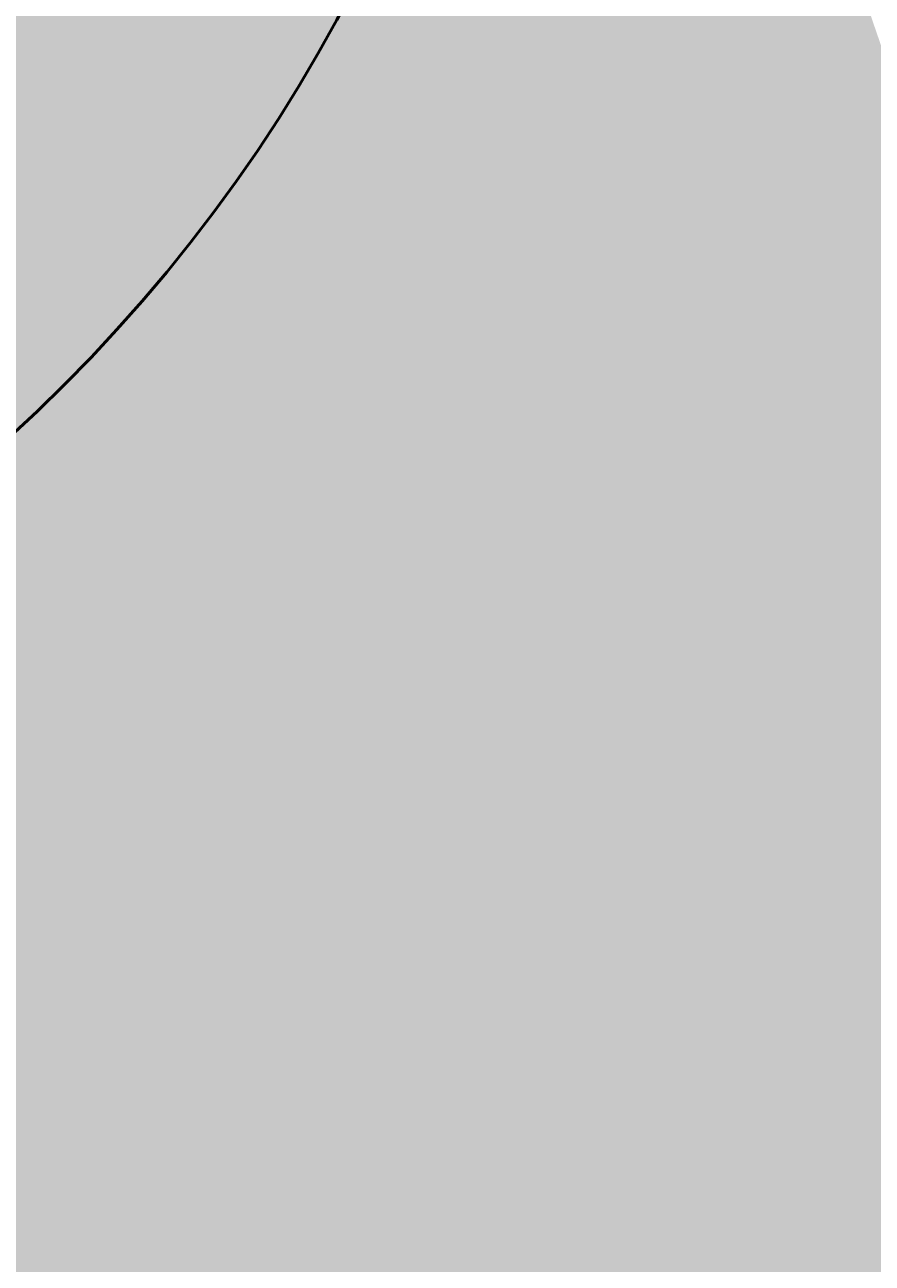
# Model space of a CAD drawing. Units: inches. Extents: x 114 to 236, y -51 to 115.
# Tile 10 of 14: x 196 to 212, y 41 to 65. Entities that reach past the tile are written whole.
import ezdxf

# ---------------------------------------------------------------- set-up
doc = ezdxf.new("R2010")
doc.units = ezdxf.units.IN
doc.header["$MEASUREMENT"] = 0
doc.layers.add('M-DIMS', color=2, linetype='Continuous', lineweight=18)
doc.layers.add('M-OUTL', color=7, linetype='Continuous', lineweight=50)
doc.layers.add('M-HATC', color=7, linetype='Continuous', lineweight=18, true_color=0xffffff)
doc.styles.get("Standard").update_dxf_attribs({"font": 'arial.ttf'})
doc.dimstyles.get("Standard").update_dxf_attribs({"dimtxt": 0.18, "dimasz": 0.18, "dimexe": 0.18, "dimexo": 0.0625, "dimgap": 0.09, "dimtad": 0, "dimtih": 1, "dimtoh": 1, "dimdec": 4, "dimzin": 0, "dimdsep": 46, "dimtxsty": 'Standard', "dimcen": 0.09, "dimadec": 0, "dimazin": 0, "dimtfac": 1, "dimtdec": 4, "dimtofl": 0, "dimtmove": 0, "dimatfit": 3, "dimfxl": 1, "dimtolj": 1, "dimtzin": 0, "dimarcsym": 0})

# ---------------------------------------------------------------- blocks, each defined once
blk = doc.blocks.new('*D3')
at = {"layer": 'Defpoints', "color": 0, "transparency": 16777216}
for p in [(230.229, 115.287), (120.229, 9.307), (230.229, 9.307)]:
    blk.add_point(p, dxfattribs=at)
at = {"layer": 'M-DIMS', "color": 0, "lineweight": -2, "transparency": 16777216}
for p, q in [((120.229, 9.37), (120.229, 115.467)), ((120.409, 115.287), (174.949, 115.287)), ((230.049, 115.287), (175.509, 115.287)), ((230.229, 9.37), (230.229, 115.467))]:
    blk.add_line(p, q, dxfattribs=at)
at = {"layer": 'M-DIMS', "color": 0, "transparency": 16777216}
for points in [[(120.409, 115.317), (120.409, 115.257), (120.229, 115.287)], [(230.049, 115.317), (230.049, 115.257), (230.229, 115.287)]]:
    blk.add_solid(points, dxfattribs=at)
at = {"layer": 'M-DIMS', "color": 0, "transparency": 16777216, "insert": (175.229, 115.287), "char_height": 0.18, "attachment_point": 5}
blk.add_mtext('\\A1;110', dxfattribs=at)
blk = doc.blocks.new('*D6')
at = {"layer": 'Defpoints', "color": 0, "transparency": 16777216}
for p in [(175.229, 79.307), (215.229, 9.307), (215.229, -11.673)]:
    blk.add_point(p, dxfattribs=at)
at = {"layer": 'M-DIMS', "color": 0, "lineweight": -2, "transparency": 16777216}
for p, q in [((175.229, 79.245), (175.229, -11.853)), ((215.229, 9.245), (215.229, -11.853)), ((175.409, -11.673), (195.006, -11.673)), ((215.049, -11.673), (195.451, -11.673))]:
    blk.add_line(p, q, dxfattribs=at)
at = {"layer": 'M-DIMS', "color": 0, "transparency": 16777216}
for points in [[(175.409, -11.643), (175.409, -11.703), (175.229, -11.673)], [(215.049, -11.643), (215.049, -11.703), (215.229, -11.673)]]:
    blk.add_solid(points, dxfattribs=at)
at = {"layer": 'M-DIMS', "color": 0, "transparency": 16777216, "insert": (195.229, -11.673), "char_height": 0.18, "attachment_point": 5}
blk.add_mtext('\\A1;40', dxfattribs=at)
blk = doc.blocks.new('*D7')
at = {"layer": 'Defpoints', "color": 0, "transparency": 16777216}
for p in [(175.229, 79.307), (236.209, 79.307), (215.229, 9.307)]:
    blk.add_point(p, dxfattribs=at)
at = {"layer": 'M-DIMS', "color": 0, "lineweight": -2, "transparency": 16777216}
for p, q in [((175.291, 79.307), (236.389, 79.307)), ((236.209, 79.127), (236.209, 44.489)), ((236.209, 9.487), (236.209, 44.125)), ((215.291, 9.307), (236.389, 9.307))]:
    blk.add_line(p, q, dxfattribs=at)
at = {"layer": 'M-DIMS', "color": 0, "transparency": 16777216}
for points in [[(236.179, 79.127), (236.239, 79.127), (236.209, 79.307)], [(236.179, 9.487), (236.239, 9.487), (236.209, 9.307)]]:
    blk.add_solid(points, dxfattribs=at)
at = {"layer": 'M-DIMS', "color": 0, "transparency": 16777216, "insert": (236.209, 44.307), "char_height": 0.18, "attachment_point": 5}
blk.add_mtext('\\A1;70', dxfattribs=at)
blk = doc.blocks.new('*D8')
at = {"layer": 'Defpoints', "color": 0, "transparency": 16777216}
for p in [(197.149, 99.789), (153.308, 58.825)]:
    blk.add_point(p, dxfattribs=at)
at = {"layer": 'M-DIMS', "color": 0, "lineweight": -2, "transparency": 16777216}
for p, q in [((210.301, 112.078), (197.28, 99.912)), ((210.481, 112.078), (210.301, 112.078)), ((175.229, 79.217), (175.229, 79.397)), ((175.139, 79.307), (175.319, 79.307))]:
    blk.add_line(p, q, dxfattribs=at)
at = {"layer": 'M-DIMS', "color": 0, "transparency": 16777216}
blk.add_solid([(197.26, 99.934), (197.301, 99.89), (197.149, 99.789)], dxfattribs=at)
at = {"layer": 'M-DIMS', "color": 0, "transparency": 16777216, "insert": (210.797, 112.078), "char_height": 0.18, "attachment_point": 5}
blk.add_mtext('\\A1;∅60', dxfattribs=at)

msp = doc.modelspace()

# ---------------------------------------------------------------- hatches: boundary and pattern name
at = {"layer": 'M-HATC'}
h = msp.add_hatch(color=256, dxfattribs=at)
h.set_gradient(color1=(19, 155, 72), color2=(255, 255, 0), tint=1, name='HEMISPHERICAL')
h.paths.add_polyline_path([(147.853, 91.577), (146.105, 86.505, 0.060651), (145.229, 79.307, 1), (205.229, 79.307, 0.060651), (204.352, 86.505), (202.605, 91.577, 0.647643)])
h.paths.add_polyline_path([(180.229, 99.307, -0.031342), (180.189, 98.682, -0.27393), (194.604, 84.268, -0.451416), (200.229, 79.307, -0.451416), (194.604, 74.346, -0.27393), (180.189, 59.932, -0.031342), (180.229, 59.307, -1), (170.229, 59.307, -0.031342), (170.268, 59.932, -0.27393), (155.854, 74.346, -0.451416), (150.229, 79.307, -0.451416), (155.854, 84.268, -0.27393), (170.268, 98.682, -0.031342), (170.229, 99.307, -1)], flags=16)
h.paths.add_polyline_path([(183.229, 79.307, -1), (167.229, 79.307, -1)], flags=0)
h.paths.add_polyline_path([(155.854, 84.268, -0.377964), (160.229, 79.307, -0.377964), (155.854, 74.346, 0.27393), (170.268, 59.932, -0.881917), (180.189, 59.932, 0.27393), (194.604, 74.346, -0.377964), (190.229, 79.307, -0.377964), (194.604, 84.268, 0.27393), (180.189, 98.682, -0.881917), (170.268, 98.682, 0.27393)], flags=0)
h = msp.add_hatch(color=256, dxfattribs=at)
h.set_gradient(color1=(242, 103, 34), color2=(255, 255, 0), tint=1, name='INVSPHERICAL')
h.paths.add_polyline_path([(145.229, 79.307, -0.060651), (146.105, 86.505), (121.823, 16.038, -0.790743), (150.229, 9.307, -0.236068), (144.229, -2.693, -0.14094), (175.229, 9.098, -0.14094), (206.229, -2.693, -0.236068), (200.229, 9.307, -0.790743), (228.634, 16.038), (204.352, 86.505, -0.060651), (205.229, 79.307, -1)])

# ---------------------------------------------------------------- linework, layer by layer
at = {"layer": 'M-OUTL'}
msp.add_circle((175.229, 79.307), 30, dxfattribs=at)

# ---------------------------------------------------------------- dimensions: what is measured, and where the dimension line sits
at = {"layer": 'M-DIMS'}
for base, p1, p2, picture, middle in [((230.229, 115.287), (120.229, 9.307), (230.229, 9.307), '*D3', (175.229, 115.287)), ((215.229, -11.673), (175.229, 79.307), (215.229, 9.307), '*D6', (195.229, -11.673))]:
    dim = msp.add_linear_dim(base=base, p1=p1, p2=p2, dimstyle='Standard', override={"dimdec": 0, "dimlfac": 1, "dimrnd": 0, "dimzin": 0, "dimdsep": 46, "dimlunit": 2}, dxfattribs=at)
    dim.commit()
    dim.dimension.update_dxf_attribs({"geometry": picture, "text_midpoint": middle})
dim = msp.add_diameter_dim_2p(p1=(153.308, 58.825), p2=(197.149, 99.789), dimstyle='Standard', override={"dimdec": 0, "dimlfac": 1, "dimrnd": 0, "dimzin": 0, "dimdsep": 46, "dimlunit": 2}, dxfattribs=at)
dim.commit()
dim.dimension.update_dxf_attribs({"geometry": '*D8', "text_midpoint": (210.797, 112.078), "dimtype": 163})
dim = msp.add_linear_dim(base=(236.209, 79.307), p1=(215.229, 9.307), p2=(175.229, 79.307), angle=90, dimstyle='Standard', override={"dimdec": 0, "dimlfac": 1, "dimrnd": 0, "dimzin": 0, "dimdsep": 46, "dimlunit": 2}, dxfattribs=at)
dim.commit()
dim.dimension.update_dxf_attribs({"geometry": '*D7', "text_midpoint": (236.209, 44.307)})

doc.saveas('drawing.dxf')
